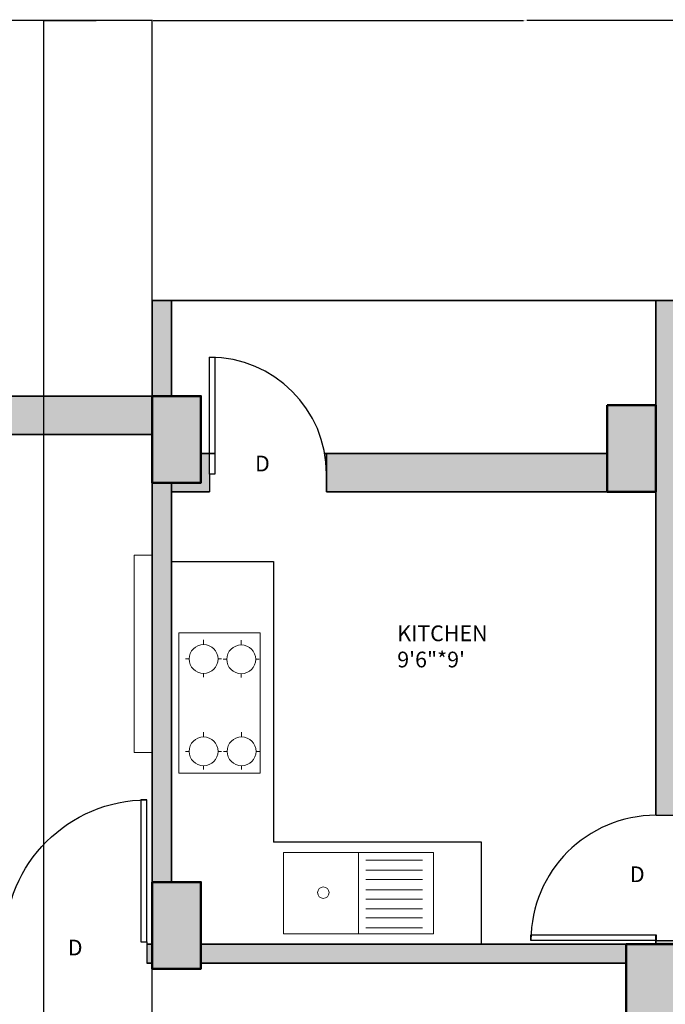
# Model space of a CAD drawing. Units: inches. Extents: x 1998 to 2588, y 1139 to 1977.
# Tile 76 of 134: x 2192 to 2344, y 1746 to 1977. Entities that reach past the tile are written whole.
import ezdxf

# ---------------------------------------------------------------- set-up
doc = ezdxf.new("R2010")
doc.units = ezdxf.units.IN
for name, color, linetype, lineweight in [('A-ANNO-DIMS', 2, 'Continuous', 18), ('A-AREA-IDEN', 7, 'Continuous', 18), ('A-COLS-PATT', 250, 'Continuous', 13), ('A-DOOR-IDEN', 7, 'Continuous', 18), ('A-EQPM', 21, 'Continuous', 18), ('A-FLOR-CASE', 32, 'Continuous', 25), ('A-FLOR-FIXT', 9, 'Continuous', 18), ('A-WALL-PATT', 252, 'Continuous', 13), ('COLUMN', 10, 'Continuous', 50), ('DOOR', 52, 'Continuous', 25), ('FUR', 21, 'Continuous', 18), ('WALL', 200, 'Continuous', 35)]:
    doc.layers.add(name, color=color, linetype=linetype, lineweight=lineweight)
doc.styles.get("Standard").update_dxf_attribs({"font": 'arial.ttf'})
doc.dimstyles.get("Standard").update_dxf_attribs({"dimtxt": 0.18, "dimasz": 0.18, "dimexe": 0.18, "dimexo": 0.0625, "dimgap": 0.09, "dimtad": 0, "dimtih": 1, "dimtoh": 1, "dimdec": 4, "dimzin": 0, "dimdsep": 46, "dimtxsty": 'Standard', "dimcen": 0.09, "dimadec": 0, "dimazin": 0, "dimtfac": 1, "dimtdec": 4, "dimtofl": 0, "dimtmove": 0, "dimatfit": 3, "dimfxl": 1, "dimtolj": 1, "dimtzin": 0, "dimarcsym": 0})

# ---------------------------------------------------------------- blocks, each defined once
blk = doc.blocks.new('*U2')
for p, q in [((0, 0), (0, -6)), ((40, 0), (40, -6))]:
    blk.add_line(p, q)
blk.add_lwpolyline([(0, 0), (0, 40), (1.75, 40), (1.75, 0)], close=True)
blk.add_arc((0, 0), 40, 0, 90)
blk = doc.blocks.new('*D25')
at = {"layer": 'A-ANNO-DIMS', "color": 0, "lineweight": -2, "transparency": 16777216}
for p, q in [((2087.97, 1888.79), (2087.97, 1977.36)), ((2088.15, 1977.18), (2155.19, 1977.18)), ((2222.79, 1977.18), (2155.75, 1977.18)), ((2222.97, 1888.79), (2222.97, 1977.36))]:
    blk.add_line(p, q, dxfattribs=at)
at = {"layer": 'A-ANNO-DIMS', "color": 0, "transparency": 16777216}
for points in [[(2088.15, 1977.21), (2088.15, 1977.15), (2087.97, 1977.18)], [(2222.79, 1977.21), (2222.79, 1977.15), (2222.97, 1977.18)]]:
    blk.add_solid(points, dxfattribs=at)
at = {"layer": 'Defpoints', "color": 0, "transparency": 16777216}
for p in [(2222.97, 1977.18), (2087.97, 1888.73), (2222.97, 1888.73)]:
    blk.add_point(p, dxfattribs=at)
at = {"layer": 'A-ANNO-DIMS', "color": 0, "transparency": 16777216, "insert": (2155.47, 1977.18), "char_height": 0.18, "attachment_point": 5}
blk.add_mtext('\\A1;135', dxfattribs=at)
blk = doc.blocks.new('*D26')
at = {"layer": 'A-ANNO-DIMS', "color": 0, "lineweight": -2, "transparency": 16777216}
for p, q in [((2222.97, 1911.29), (2222.97, 1977.36)), ((2223.15, 1977.18), (2310.34, 1977.18)), ((2398.29, 1977.18), (2311.11, 1977.18)), ((2398.47, 1911.29), (2398.47, 1977.36))]:
    blk.add_line(p, q, dxfattribs=at)
at = {"layer": 'A-ANNO-DIMS', "color": 0, "transparency": 16777216}
for points in [[(2223.15, 1977.21), (2223.15, 1977.15), (2222.97, 1977.18)], [(2398.29, 1977.21), (2398.29, 1977.15), (2398.47, 1977.18)]]:
    blk.add_solid(points, dxfattribs=at)
at = {"layer": 'Defpoints', "color": 0, "transparency": 16777216}
for p in [(2398.47, 1977.18), (2222.97, 1911.23), (2398.47, 1911.23)]:
    blk.add_point(p, dxfattribs=at)
at = {"layer": 'A-ANNO-DIMS', "color": 0, "transparency": 16777216, "insert": (2310.72, 1977.18), "char_height": 0.18, "attachment_point": 5}
blk.add_mtext('\\A1;175.5', dxfattribs=at)
blk = doc.blocks.new('*D36')
at = {"layer": 'A-ANNO-DIMS', "color": 0, "lineweight": -2, "transparency": 16777216}
for p, q in [((2197.45, 1663.31), (2197.45, 1977.36)), ((2197.63, 1977.18), (2209.75, 1977.18)), ((2222.79, 1977.18), (2210.68, 1977.18)), ((2222.97, 1663.31), (2222.97, 1977.36))]:
    blk.add_line(p, q, dxfattribs=at)
at = {"layer": 'A-ANNO-DIMS', "color": 0, "transparency": 16777216}
for points in [[(2197.63, 1977.21), (2197.63, 1977.15), (2197.45, 1977.18)], [(2222.79, 1977.21), (2222.79, 1977.15), (2222.97, 1977.18)]]:
    blk.add_solid(points, dxfattribs=at)
at = {"layer": 'Defpoints', "color": 0, "transparency": 16777216}
for p in [(2222.97, 1977.18), (2197.45, 1663.25), (2222.97, 1663.25)]:
    blk.add_point(p, dxfattribs=at)
at = {"layer": 'A-ANNO-DIMS', "color": 0, "transparency": 16777216, "insert": (2210.21, 1977.18), "char_height": 0.18, "attachment_point": 5}
blk.add_mtext('\\A1;25.523', dxfattribs=at)
blk = doc.blocks.new('*D37')
at = {"layer": 'A-ANNO-DIMS', "color": 0, "lineweight": -2, "transparency": 16777216}
for p, q in [((2148.45, 1612.79), (2148.45, 1977.36)), ((2148.63, 1977.18), (2172.73, 1977.18)), ((2197.27, 1977.18), (2173.18, 1977.18)), ((2197.45, 1612.79), (2197.45, 1977.36))]:
    blk.add_line(p, q, dxfattribs=at)
at = {"layer": 'A-ANNO-DIMS', "color": 0, "transparency": 16777216}
for points in [[(2148.63, 1977.21), (2148.63, 1977.15), (2148.45, 1977.18)], [(2197.27, 1977.21), (2197.27, 1977.15), (2197.45, 1977.18)]]:
    blk.add_solid(points, dxfattribs=at)
at = {"layer": 'Defpoints', "color": 0, "transparency": 16777216}
for p in [(2197.45, 1977.18), (2148.45, 1612.73), (2197.45, 1612.73)]:
    blk.add_point(p, dxfattribs=at)
at = {"layer": 'A-ANNO-DIMS', "color": 0, "transparency": 16777216, "insert": (2172.95, 1977.18), "char_height": 0.18, "attachment_point": 5}
blk.add_mtext('\\A1;49', dxfattribs=at)

msp = doc.modelspace()

# ---------------------------------------------------------------- hatches: boundary and pattern name
at = {"layer": 'A-COLS-PATT'}
h = msp.add_hatch(color=256, dxfattribs=at)
h.dxf.hatch_style = 1
h.paths.add_polyline_path([(2099.4125, 1888.7324), (2087.9729, 1888.7324), (2087.9729, 1868.3278), (2099.4125, 1868.3278)])
h.paths.add_polyline_path([(2234.4125, 1888.7324), (2222.9729, 1888.7324), (2222.9729, 1868.3278), (2234.4125, 1868.3278)])
h.paths.add_polyline_path([(2341.4729, 1886.637), (2330.0332, 1886.637), (2330.0332, 1866.2324), (2341.4729, 1866.2324)])
h.paths.add_polyline_path([(2507.8006, 1882.7324), (2487.396, 1882.7324), (2487.396, 1871.2927), (2507.8006, 1871.2927)])
h.paths.add_polyline_path([(2510.9729, 1766.672), (2490.5682, 1766.672), (2490.5682, 1755.2324), (2510.9729, 1755.2324)])
h.paths.add_polyline_path([(2345.9729, 1759.7324), (2334.5332, 1759.7324), (2334.5332, 1739.3278), (2345.9729, 1739.3278)])
h.paths.add_polyline_path([(2234.4125, 1774.3318), (2222.9729, 1774.3318), (2222.9729, 1753.9272), (2234.4125, 1753.9272)])
h.paths.add_polyline_path([(2099.4125, 1775.637), (2087.9729, 1775.637), (2087.9729, 1755.2324), (2099.4125, 1755.2324)])
h.paths.add_polyline_path([(2098.0956, 1593.7241), (2077.691, 1593.7241), (2077.691, 1582.2845), (2098.0956, 1582.2845)])
h.paths.add_polyline_path([(2227.4729, 1604.637), (2216.0332, 1604.637), (2216.0332, 1584.2324), (2227.4729, 1584.2324)])
h.paths.add_polyline_path([(2345.9729, 1647.5211), (2334.5332, 1647.5211), (2334.5332, 1627.1165), (2345.9729, 1627.1165)])
h.paths.add_polyline_path([(2522.3775, 1641.2324), (2501.9729, 1641.2324), (2501.9729, 1629.7927), (2522.3775, 1629.7927)])
h.paths.add_polyline_path([(2522.3775, 1480.7324), (2501.9729, 1480.7324), (2501.9729, 1469.2927), (2522.3775, 1469.2927)])
h.paths.add_polyline_path([(2345.9729, 1488.5616), (2334.5332, 1488.5616), (2334.5332, 1468.1569), (2345.9729, 1468.1569)])
h.paths.add_polyline_path([(2234.4125, 1486.137), (2227.4729, 1486.137), (2227.4729, 1465.7324), (2234.4125, 1465.7324)])
h.paths.add_polyline_path([(2227.4729, 1486.137), (2222.9729, 1486.137), (2222.9729, 1465.7324), (2227.4729, 1465.7324)])
h.paths.add_polyline_path([(2108.3775, 1470.2324), (2087.9729, 1470.2324), (2087.9729, 1458.7927), (2108.3775, 1458.7927)])
h.paths.add_polyline_path([(2096.9729, 1365.5012), (2087.9729, 1365.5012), (2087.9729, 1345.0966), (2096.9729, 1345.0966)])
h.paths.add_polyline_path([(2087.9729, 1365.5012), (2085.5332, 1365.5012), (2085.5332, 1345.0966), (2087.9729, 1345.0966)])
h.paths.add_polyline_path([(2234.4125, 1285.137), (2222.9729, 1285.137), (2222.9729, 1264.7324), (2234.4125, 1264.7324)])
h.paths.add_polyline_path([(2345.9729, 1285.137), (2334.5332, 1285.137), (2334.5332, 1264.7324), (2345.9729, 1264.7324)])
h.paths.add_polyline_path([(2503.1458, 1240.172), (2482.7412, 1240.172), (2482.7412, 1228.7324), (2503.1458, 1228.7324)])
h.paths.add_polyline_path([(2510.9729, 1369.172), (2490.5682, 1369.172), (2490.5682, 1357.7324), (2510.9729, 1357.7324)])
at = {"layer": 'A-WALL-PATT'}
h = msp.add_hatch(color=256, dxfattribs=at)
h.dxf.hatch_style = 1
h.paths.add_polyline_path([(2227.4729, 1911.2324), (2222.9729, 1911.2324), (2222.9729, 1888.7324), (2227.4729, 1888.7324)])
h.paths.add_polyline_path([(2236.4493, 1870.3636), (2236.4493, 1875.2324), (2234.4125, 1875.2324), (2234.4125, 1868.3278), (2227.4729, 1868.3278), (2227.4729, 1866.2324), (2236.4493, 1866.2324)])
h.paths.add_polyline_path([(2330.0332, 1875.2324), (2263.9907, 1875.2324), (2263.9907, 1866.2324), (2330.0332, 1866.2324)])
h.paths.add_polyline_path([(2345.9729, 1906.7324), (2393.9729, 1906.7324), (2393.9729, 1882.7324), (2345.9729, 1882.7324), (2345.9729, 1878.2324), (2393.9729, 1878.2324), (2398.4729, 1878.2324), (2398.4729, 1882.7324), (2398.4729, 1911.2324), (2345.9729, 1911.2324), (2341.4729, 1911.2324), (2341.4729, 1866.2324), (2341.4729, 1790.0412), (2345.9729, 1790.0412), (2345.9729, 1875.2324)])
h.paths.add_polyline_path([(2398.4729, 1878.2324), (2393.9729, 1878.2324), (2393.9729, 1798.2324), (2393.9729, 1793.7324), (2398.4729, 1793.7324)], flags=17)
h.paths.add_polyline_path([(2393.9729, 1798.2324), (2375.7311, 1798.2324, -0.00596797), (2375.7384, 1797.6146), (2375.7384, 1793.7324), (2393.9729, 1793.7324)], flags=17)
h.paths.add_polyline_path([(2349.8569, 1797.6146), (2349.8569, 1798.2324), (2345.9729, 1798.2324), (2345.9729, 1793.7324), (2349.8569, 1793.7324)], flags=17)
h.paths.add_polyline_path([(2398.4729, 1793.7324), (2393.9729, 1793.7324), (2393.9729, 1790.0412), (2398.4729, 1790.0412)], flags=17)
h.paths.add_polyline_path([(2527.4729, 1882.7324), (2507.8006, 1882.7324), (2507.8006, 1878.2324), (2518.4729, 1878.2324), (2518.4729, 1759.7324), (2510.9729, 1759.7324), (2510.9729, 1755.2324), (2527.4729, 1755.2324)])
h.paths.add_polyline_path([(2487.396, 1882.7324), (2398.4729, 1882.7324), (2398.4729, 1878.2324), (2487.396, 1878.2324)])
h.paths.add_polyline_path([(2490.5682, 1759.7324), (2345.9729, 1759.7324), (2345.9729, 1755.2324), (2490.5682, 1755.2324)])
h.paths.add_polyline_path([(2398.4729, 1760.5844), (2398.3914, 1760.5844), (2393.9729, 1760.5844), (2393.9729, 1759.7324), (2398.4729, 1759.7324)])
h.paths.add_polyline_path([(2334.5332, 1759.7324), (2234.4125, 1759.7324), (2234.4125, 1755.2324), (2334.5332, 1755.2324)])
h.paths.add_polyline_path([(2345.9729, 1760.5844), (2341.5543, 1760.5844), (2341.4729, 1760.5844), (2341.4729, 1759.7324), (2345.9729, 1759.7324)])
h.paths.add_polyline_path([(2222.9729, 1759.7324), (2221.7204, 1759.7324), (2221.7204, 1755.2324), (2222.9729, 1755.2324)])
h.paths.add_polyline_path([(2061.4729, 1702.7324), (2059.4729, 1702.7324), (2059.4729, 1584.2324), (2061.4729, 1584.2324)])
h.paths.add_polyline_path([(2061.4729, 1584.2324), (2059.4729, 1584.2324), (2059.4729, 1470.2324), (2061.4729, 1470.2324)])
h.paths.add_polyline_path([(2510.9729, 1469.2927), (2501.9729, 1469.2927), (2501.9729, 1369.172), (2510.9729, 1369.172)])
h.paths.add_polyline_path([(2227.4729, 1369.7324), (2227.4729, 1417.7324), (2221.4126, 1417.7324), (2221.4126, 1413.2324), (2222.9729, 1413.2324), (2222.9729, 1293.2324), (2222.9729, 1285.137), (2227.4729, 1285.137)])
h = msp.add_hatch(color=256, dxfattribs=at)
h.dxf.hatch_style = 1
h.paths.add_polyline_path([(2222.9729, 1888.7324), (2099.4125, 1888.7324), (2099.4125, 1879.7324), (2222.9729, 1879.7324)])
h.paths.add_polyline_path([(2096.9729, 1868.3278), (2087.9729, 1868.3278), (2087.9729, 1775.637), (2096.9729, 1775.637)])
h.paths.add_polyline_path([(2227.4729, 1868.3278), (2222.9729, 1868.3278), (2222.9729, 1774.3318), (2227.4729, 1774.3318)])
h.paths.add_polyline_path([(2188.3019, 1759.7324), (2138.6074, 1759.7324), (2099.4125, 1759.7324), (2099.4125, 1755.2324), (2176.9729, 1755.2324), (2188.3019, 1755.2324)])
h.paths.add_polyline_path([(2087.9729, 1759.7324), (2059.4729, 1759.7324), (2059.4729, 1702.7324), (2087.9729, 1702.7324), (2087.9729, 1707.2324), (2063.9729, 1707.2324), (2063.9729, 1755.2324), (2087.9729, 1755.2324)])
h.paths.add_polyline_path([(2096.9729, 1755.2324), (2087.9729, 1755.2324), (2087.9729, 1707.2324), (2096.9729, 1707.2324)])
h.paths.add_polyline_path([(2187.0461, 1707.2324), (2105.9729, 1707.2324), (2096.9729, 1707.2324), (2087.9729, 1707.2324), (2087.9729, 1702.7324), (2105.9729, 1702.7324), (2114.9729, 1702.7324), (2187.0461, 1702.7324)])
h.paths.add_polyline_path([(2181.4729, 1719.2028), (2176.9729, 1719.2028), (2176.9729, 1707.2324), (2181.4729, 1707.2324)])
h.paths.add_polyline_path([(2216.0332, 1588.7324), (2114.9729, 1588.7324), (2105.9729, 1588.7324), (2105.9729, 1584.2324), (2216.0332, 1584.2324)])
h.paths.add_polyline_path([(2077.691, 1588.7324), (2061.4729, 1588.7324), (2061.4729, 1584.2324), (2077.691, 1584.2324)])
h.paths.add_polyline_path([(2105.9729, 1588.7324), (2098.0956, 1588.7324), (2098.0956, 1584.2324), (2105.9729, 1584.2324)])
h.paths.add_polyline_path([(2114.9729, 1596.2642), (2110.1012, 1596.2642), (2105.9729, 1596.2642), (2105.9729, 1588.7324), (2114.9729, 1588.7324)])
h.paths.add_polyline_path([(2114.9729, 1584.2324), (2105.9729, 1584.2324), (2105.9729, 1580.249), (2110.1012, 1580.249), (2114.9729, 1580.249)])
h.paths.add_polyline_path([(2114.9729, 1547.7716), (2110.1012, 1547.7716, -0.0318759), (2105.9729, 1548.035), (2105.9729, 1470.2324), (2108.3775, 1470.2324), (2108.3775, 1465.7324), (2186.2943, 1465.7324), (2186.2943, 1470.2324), (2114.9729, 1470.2324)])
h.paths.add_polyline_path([(2227.4729, 1584.2324), (2222.9729, 1584.2324), (2222.9729, 1486.137), (2227.4729, 1486.137)])
h.paths.add_polyline_path([(2295.4138, 1593.2324), (2227.4729, 1593.2324), (2227.4729, 1588.7324), (2295.4138, 1588.7324), (2295.4138, 1591.8729)])
h.paths.add_polyline_path([(2345.9729, 1627.1165), (2341.4729, 1627.1165), (2341.4729, 1593.2324), (2337.2869, 1593.2324), (2337.2869, 1591.8729), (2337.2869, 1588.7324), (2345.9729, 1588.7324)])
h.paths.add_polyline_path([(2291.9729, 1588.7324), (2287.4729, 1588.7324), (2287.4729, 1522.7324), (2291.9729, 1522.7324)])
h.paths.add_polyline_path([(2291.9729, 1522.7324), (2287.4729, 1522.7324), (2227.4729, 1522.7324), (2227.4729, 1518.2324), (2291.9729, 1518.2324)])
h.paths.add_polyline_path([(2295.7347, 1519.5919), (2295.7347, 1522.7324), (2291.9729, 1522.7324), (2291.9729, 1518.2324), (2295.7347, 1518.2324)])
h.paths.add_polyline_path([(2345.9729, 1522.7324), (2337.6078, 1522.7324), (2337.6078, 1519.5919), (2337.6078, 1518.2324), (2341.4729, 1518.2324), (2341.4729, 1488.5616), (2345.9729, 1488.5616)])
h.paths.add_polyline_path([(2345.9729, 1468.1569), (2341.4729, 1468.1569), (2341.4729, 1374.2324), (2227.4729, 1374.2324), (2227.4729, 1369.7324), (2345.9729, 1369.7324)])
h.paths.add_polyline_path([(2345.9729, 1369.7324), (2341.4729, 1369.7324), (2341.4729, 1362.2324), (2345.9729, 1362.2324)])
h.paths.add_polyline_path([(2345.9729, 1317.7324), (2345.9729, 1322.2324), (2341.4729, 1322.2324), (2341.4729, 1285.137), (2345.9729, 1285.137)], flags=17)
h.paths.add_polyline_path([(2356.2096, 1322.2324), (2345.9729, 1322.2324), (2345.9729, 1317.7324), (2356.2096, 1317.7324), (2356.2096, 1319.3088)], flags=17)
h.paths.add_polyline_path([(2393.9729, 1322.2324), (2375.6999, 1322.2324), (2375.6999, 1319.3088, -0.02024576), (2375.636, 1317.7324), (2393.9729, 1317.7324)], flags=17)
h.paths.add_polyline_path([(2398.4729, 1322.2324), (2393.9729, 1322.2324), (2393.9729, 1317.7324), (2393.9729, 1237.7324), (2345.9729, 1237.7324), (2345.9729, 1264.7324), (2341.4729, 1264.7324), (2341.4729, 1228.7324), (2393.9729, 1228.7324), (2482.7412, 1228.7324), (2482.7412, 1237.7324), (2398.4729, 1237.7324), (2398.4729, 1297.1029)])
h.paths.add_polyline_path([(2398.4729, 1362.2324), (2393.9729, 1362.2324), (2393.9729, 1357.7324), (2398.4729, 1357.7324)])
h.paths.add_polyline_path([(2345.9729, 1329.7549), (2341.4729, 1329.7549), (2341.4729, 1322.2324), (2345.9729, 1322.2324)])

# ---------------------------------------------------------------- linework, layer by layer
at = {"layer": 'A-EQPM'}
for p, q in [((2235.0461, 1830.2466), (2235.0461, 1831.355)), ((2243.9199, 1830.1663), (2243.9199, 1831.2748)), ((2231.6454, 1826.8458), (2230.8032, 1826.8458)), ((2238.4468, 1826.8458), (2239.2734, 1826.8458)), ((2240.5192, 1826.7656), (2239.677, 1826.7656)), ((2247.3206, 1826.7656), (2248.1472, 1826.7656)), ((2235.0461, 1823.4451), (2235.0461, 1822.5616)), ((2243.9199, 1823.3648), (2243.9199, 1822.4813)), ((2235.0461, 1808.5038), (2235.0461, 1809.6123)), ((2243.9943, 1808.5038), (2243.9943, 1809.6123)), ((2231.6454, 1805.1031), (2230.8032, 1805.1031)), ((2238.4468, 1805.1031), (2239.2734, 1805.1031)), ((2240.5936, 1805.1031), (2239.7514, 1805.1031)), ((2247.3951, 1805.1031), (2248.2216, 1805.1031)), ((2235.0461, 1801.7024), (2235.0461, 1800.8188)), ((2243.9943, 1801.7024), (2243.9943, 1800.8188))]:
    msp.add_line(p, q, dxfattribs=at)
msp.add_lwpolyline([(2229.2287, 1833.0068), (2248.3942, 1833.0068), (2248.3942, 1799.9263), (2229.2287, 1799.9263)], close=True, dxfattribs=at)
for centre in [(2235.0461, 1826.8458), (2243.9199, 1826.7656), (2235.0461, 1805.1031), (2243.9943, 1805.1031)]:
    msp.add_circle(centre, 3.4007, dxfattribs=at)
at = {"layer": 'A-FLOR-CASE'}
for p, q in [((2227.4729, 1849.7738), (2251.4729, 1849.7738)), ((2251.4729, 1849.7738), (2251.4729, 1783.7324)), ((2300.468, 1783.7324), (2251.4729, 1783.7324)), ((2300.468, 1759.7324), (2300.468, 1783.7324))]:
    msp.add_line(p, q, dxfattribs=at)
at = {"layer": 'A-FLOR-FIXT'}
for p, q in [((2271.5332, 1762.1193), (2271.5332, 1781.2935)), ((2273.2605, 1779.5103), (2286.6114, 1779.5103)), ((2273.2605, 1777.1421), (2286.6114, 1777.1421)), ((2273.2605, 1774.9672), (2286.6114, 1774.9672)), ((2273.2605, 1772.5023), (2286.6114, 1772.5023)), ((2273.2605, 1770.2617), (2286.6114, 1770.2617)), ((2273.2605, 1768.0176), (2286.6114, 1768.0176)), ((2273.2605, 1765.8711), (2286.6114, 1765.8711)), ((2273.2605, 1763.5294), (2286.6114, 1763.5294))]:
    msp.add_line(p, q, dxfattribs=at)
msp.add_lwpolyline([(2253.8803, 1781.2935), (2289.1862, 1781.2935), (2289.1862, 1762.1193), (2253.8803, 1762.1193)], close=True, dxfattribs=at)
msp.add_circle((2263.2296, 1771.8293), 1.3532, dxfattribs=at)
at = {"layer": 'COLUMN'}
for points in [[(2222.9729, 1888.7324), (2234.4125, 1888.7324), (2234.4125, 1868.3278), (2222.9729, 1868.3278)], [(2330.0332, 1886.637), (2341.4729, 1886.637), (2341.4729, 1866.2324), (2330.0332, 1866.2324)], [(2222.9729, 1774.3318), (2234.4125, 1774.3318), (2234.4125, 1753.9272), (2222.9729, 1753.9272)], [(2334.5332, 1759.7324), (2345.9729, 1759.7324), (2345.9729, 1739.3278), (2334.5332, 1739.3278)]]:
    msp.add_lwpolyline(points, close=True, dxfattribs=at)
at = {"layer": 'FUR'}
msp.add_lwpolyline([(2222.9729, 1851.2937), (2218.7438, 1851.2937), (2218.7438, 1804.8339), (2222.9729, 1804.8339)], close=True, dxfattribs=at)
at = {"layer": 'WALL'}
for p, q in [((2222.9729, 1866.2324), (2222.9729, 1911.2324)), ((2345.9729, 1911.2324), (2222.9729, 1911.2324)), ((2227.4729, 1888.7324), (2227.4729, 1911.2324)), ((2227.4729, 1911.2324), (2341.4729, 1911.2324)), ((2341.4729, 1911.2324), (2341.4729, 1866.2324)), ((2227.4729, 1888.7324), (2087.9729, 1888.7324)), ((2222.9729, 1879.7324), (2099.4125, 1879.7324)), ((2222.9729, 1759.7324), (2222.9729, 1879.7324)), ((2234.4125, 1875.2324), (2237.6542, 1875.2324)), ((2263.5569, 1875.2324), (2330.0332, 1875.2324)), ((2227.4729, 1868.3278), (2227.4729, 1774.3318)), ((2227.4729, 1774.3318), (2227.4729, 1868.3278)), ((2227.4729, 1866.2324), (2227.4729, 1774.3318)), ((2227.4729, 1866.2324), (2236.4493, 1866.2324)), ((2263.9907, 1866.2324), (2341.4729, 1866.2324)), ((2341.4729, 1790.041), (2341.4729, 1866.2324)), ((2341.4729, 1759.7324), (2341.4729, 1761.8731)), ((2221.7204, 1759.7324), (2222.9729, 1759.7324)), ((2222.9729, 1755.2324), (2222.9729, 1759.7324)), ((2234.4125, 1759.7324), (2341.4729, 1759.7324)), ((2341.4729, 1759.7324), (2490.5682, 1759.7324)), ((2222.9729, 1755.2324), (2221.7204, 1755.2324)), ((2221.7204, 1755.2324), (2222.9729, 1755.2324)), ((2234.4125, 1755.2324), (2334.5332, 1755.2324)), ((2234.4125, 1755.2324), (2334.5332, 1755.2324))]:
    msp.add_line(p, q, dxfattribs=at)
for points in [[(2222.9729, 1888.7324), (2227.4729, 1888.7324), (2227.4729, 1911.2324), (2222.9729, 1911.2324)], [(2263.9907, 1866.2324), (2330.0332, 1866.2324), (2330.0332, 1875.2324), (2263.9907, 1875.2324)]]:
    msp.add_lwpolyline(points, close=True, dxfattribs=at)

# ---------------------------------------------------------------- block references
at = {"layer": 'DOOR'}
for p, xscale, yscale, zscale in [((2236.4493, 1870.3636), 0.6885363161112715, 0.6885363161112715, 0.6885363161112715), ((2221.7204, 1760.2452), -0.8354643497673233, 0.8354643497673233, 0.8354643497673233)]:
    msp.add_blockref('*U2', p, dxfattribs=dict(at, xscale=xscale, yscale=yscale, zscale=zscale))
at = {"layer": 'DOOR', "xscale": 0.7364194310947476, "yscale": 0.7364194310947476, "zscale": 0.7364194310947476, "rotation": 90}
msp.add_blockref('*U2', (2341.5543, 1760.5844), dxfattribs=at)

# ---------------------------------------------------------------- texts
at = {"layer": 'A-AREA-IDEN', "insert": (2280.6217, 1834.7363), "char_height": 3.69875, "attachment_point": 1}
msp.add_mtext_dynamic_manual_height_columns('KITCHEN\\P9\'6"*9\'', width=110.572713, gutter_width=18.4938, heights=[0], dxfattribs=at)
at = {"layer": 'A-DOOR-IDEN', "char_height": 3.6988, "attachment_point": 1}
for insert in [(2247.1518, 1874.7041), (2335.3931, 1778.0048), (2203.0755, 1760.7486)]:
    msp.add_mtext_dynamic_manual_height_columns('D', width=110.572713, gutter_width=18.4938, heights=[0], dxfattribs=dict(at, insert=insert))

# ---------------------------------------------------------------- dimensions: what is measured, and where the dimension line sits
at = {"layer": 'A-ANNO-DIMS'}
for base, p1, p2, override, picture, middle in [((2222.9729, 1977.1824), (2087.9729, 1888.7324), (2222.9729, 1888.7324), {"dimdec": 0, "dimlfac": 1, "dimrnd": 0, "dimzin": 0, "dimdsep": 46, "dimlunit": 2}, '*D25', (2155.4729, 1977.1824)), ((2197.4499, 1977.1824), (2148.4548, 1612.7324), (2197.4499, 1612.7324), {"dimdec": 0, "dimlfac": 1, "dimrnd": 0, "dimzin": 0, "dimdsep": 46, "dimlunit": 2}, '*D37', (2172.9524, 1977.1824)), ((2222.9729, 1977.1824), (2197.4499, 1663.2466), (2222.9729, 1663.2466), {"dimdec": 3, "dimlfac": 1, "dimrnd": 0, "dimzin": 0, "dimdsep": 46, "dimlunit": 2}, '*D36', (2210.2114, 1977.1824)), ((2398.4729, 1977.1824), (2222.9729, 1911.2324), (2398.4729, 1911.2324), {"dimdec": 1, "dimlfac": 1, "dimrnd": 0, "dimzin": 0, "dimdsep": 46, "dimlunit": 2}, '*D26', (2310.7229, 1977.1824))]:
    dim = msp.add_linear_dim(base=base, p1=p1, p2=p2, dimstyle='Standard', override=override, dxfattribs=at)
    dim.commit()
    dim.dimension.update_dxf_attribs({"geometry": picture, "text_midpoint": middle})

doc.saveas('drawing.dxf')
